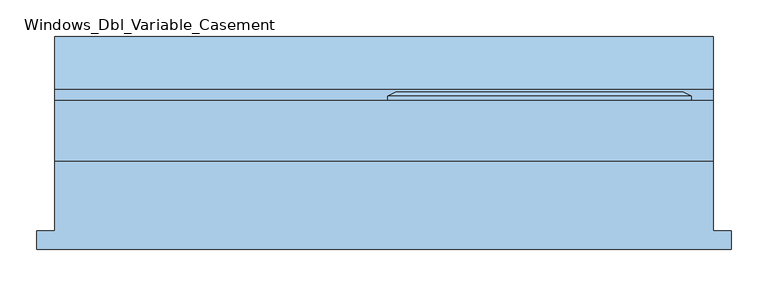
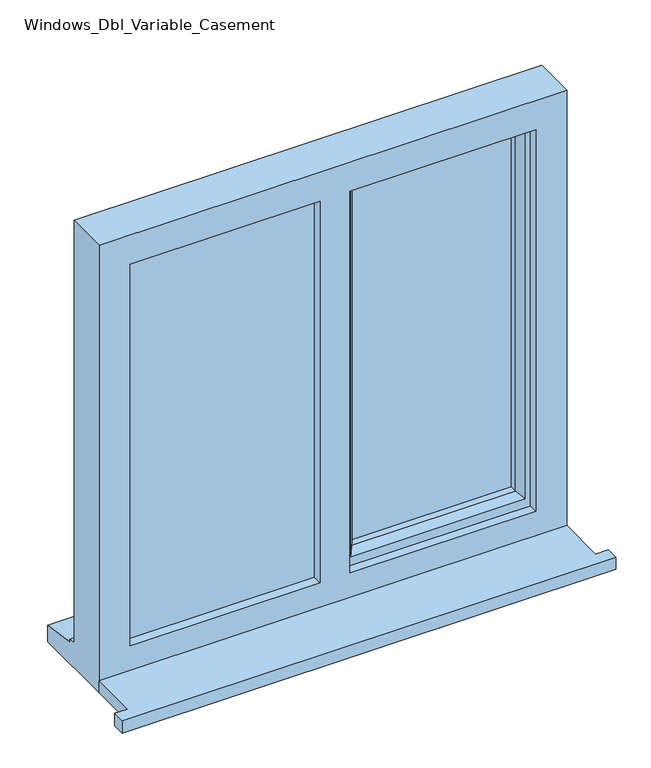
"""IFC4 building model written with IfcOpenShell, lengths in millimetres: window geometry, Windows_Dbl_Variable_Casement."""

from ifc_helpers import new_model, si_unit, frame, origin, place, context, project, spatial, polyline, outline, extrude, faceted_brep, source, transform, mapped, element, save


def windows_dbl_variable_casement_3235f540(model_context):
    return source(origin(), model_context, "Body", "SolidModel", [
        extrude(outline(polyline([(-760.0, -130.8434322), (-760.0, -105.8434322), (-735.0, -105.8434322), (-735.0, -10.2434322), (165.0, -10.2434322), (165.0, -105.8434322), (190.0, -105.8434322), (190.0, -130.8434322), (-760.0, -130.8434322)])), frame((0.0, 0.0, 1200.0), z_axis=(0.0, 0.0, 1.0), x_axis=(1.0, 0.0, 0.0)), (0.0, 0.0, 1.0), 25.0),
        faceted_brep([(-280.0, 72.7565678, 2080.0), (-280.0, 78.5300705, 2080.0), (-280.0, 78.5300705, 1253.0), (-280.0, 72.7565678, 1253.0), (-270.0, 7.7565678, 2070.0), (-270.0, 72.7565678, 2070.0), (-270.0, 72.7565678, 1263.0), (-270.0, 7.7565678, 1263.0), (-230.0, 22.2494677, 2030.0), (-240.1480377, 7.7565678, 2040.1480377), (-240.1480377, 7.7565678, 1292.8519623), (-230.0, 22.2494677, 1303.0), (-230.0, 36.7565678, 2030.0), (-230.0, 36.7565678, 1303.0), (-240.0, 60.7565678, 2040.0), (-240.0, 36.7565678, 2040.0), (-240.0, 36.7565678, 1293.0), (-240.0, 60.7565678, 1293.0), (-230.0, 78.5300705, 2030.0), (-230.0, 60.7565678, 2030.0), (-230.0, 60.7565678, 1303.0), (-230.0, 78.5300705, 1303.0), (-247.4457548, 84.3035732, 2047.4457548), (-247.4457548, 84.3035732, 1285.5542452), (-269.2153903, 84.3035732, 2069.2153903), (-269.2153903, 84.3035732, 1263.7846097), (135.0, 78.5300705, 1253.0), (135.0, 72.7565678, 1253.0), (125.0, 72.7565678, 1263.0), (125.0, 7.7565678, 1263.0), (95.1480377, 7.7565678, 1292.8519623), (85.0, 22.2494677, 1303.0), (85.0, 36.7565678, 1303.0), (95.0, 36.7565678, 1293.0), (95.0, 60.7565678, 1293.0), (85.0, 60.7565678, 1303.0), (85.0, 78.5300705, 1303.0), (102.4457548, 84.3035732, 1285.5542452), (124.2153903, 84.3035732, 1263.7846097), (135.0, 78.5300705, 2080.0), (135.0, 72.7565678, 2080.0), (125.0, 72.7565678, 2070.0), (125.0, 7.7565678, 2070.0), (95.1480377, 7.7565678, 2040.1480377), (85.0, 22.2494677, 2030.0), (85.0, 36.7565678, 2030.0), (95.0, 36.7565678, 2040.0), (95.0, 60.7565678, 2040.0), (85.0, 60.7565678, 2030.0), (85.0, 78.5300705, 2030.0), (102.4457548, 84.3035732, 2047.4457548), (124.2153903, 84.3035732, 2069.2153903)], [[[0, 1, 2, 3]], [[4, 5, 6, 7]], [[8, 9, 10, 11]], [[12, 8, 11, 13]], [[14, 15, 16, 17]], [[18, 19, 20, 21]], [[22, 18, 21, 23]], [[1, 24, 25, 2]], [[3, 2, 26, 27]], [[7, 6, 28, 29]], [[11, 10, 30, 31]], [[13, 11, 31, 32]], [[17, 16, 33, 34]], [[21, 20, 35, 36]], [[23, 21, 36, 37]], [[2, 25, 38, 26]], [[27, 26, 39, 40]], [[29, 28, 41, 42]], [[31, 30, 43, 44]], [[32, 31, 44, 45]], [[34, 33, 46, 47]], [[36, 35, 48, 49]], [[37, 36, 49, 50]], [[26, 38, 51, 39]], [[40, 39, 1, 0]], [[3, 27, 40, 0], [5, 41, 28, 6]], [[42, 41, 5, 4]], [[7, 29, 42, 4], [9, 43, 30, 10]], [[44, 43, 9, 8]], [[45, 44, 8, 12]], [[15, 46, 33, 16], [13, 32, 45, 12]], [[47, 46, 15, 14]], [[17, 34, 47, 14], [19, 48, 35, 20]], [[49, 48, 19, 18]], [[50, 49, 18, 22]], [[24, 51, 38, 25], [23, 37, 50, 22]], [[39, 51, 24, 1]]]),
        extrude(outline(polyline([(2050.0, -310.0), (2070.0, -310.0), (2070.0, -695.0), (1263.0, -695.0), (1263.0, -310.0), (1283.0, -310.0), (1283.0, -675.0), (2050.0, -675.0), (2050.0, -310.0)])), frame((0.0, 31.7565678, 0.0), z_axis=(0.0, 1.0, 0.0), x_axis=(0.0, 0.0, 1.0)), (0.0, 0.0, 1.0), 41.0),
        faceted_brep([(165.0, -10.2434322, 2110.0), (-735.0, -10.2434322, 2110.0), (-735.0, -10.2434322, 1200.0), (165.0, -10.2434322, 1200.0), (105.0, -10.2434322, 2050.0), (105.0, -10.2434322, 1275.0), (-252.0, -10.2434322, 1275.0), (-252.0, -10.2434322, 2050.0), (-310.0, -10.2434322, 2050.0), (-310.0, -10.2434322, 1275.0), (-675.0, -10.2434322, 1275.0), (-675.0, -10.2434322, 2050.0), (-735.0, 72.7565678, 2110.0), (-735.0, 72.7565678, 1251.0), (-735.0, 87.7565678, 1249.68767), (-735.0, 87.7565678, 1244.7449676), (-735.0, 160.2565678, 1233.8088847), (-735.0, 160.2565678, 1200.0), (165.0, 72.7565678, 2110.0), (165.0, 72.7565678, 1251.0), (-695.0, 72.7565678, 2070.0), (-695.0, 72.7565678, 1263.0), (-310.0, 72.7565678, 1263.0), (-310.0, 72.7565678, 2070.0), (-270.0, 72.7565678, 2070.0), (-270.0, 72.7565678, 1263.0), (125.0, 72.7565678, 1263.0), (125.0, 72.7565678, 2070.0), (-695.0, 7.7565678, 2070.0), (-695.0, 7.7565678, 1263.0), (-300.0, 7.7565678, 2070.0), (-300.0, 7.7565678, 1263.0), (-310.0, 7.7565678, 2050.0), (-675.0, 7.7565678, 2050.0), (-675.0, 7.7565678, 1275.0), (-310.0, 7.7565678, 1275.0), (-270.0, 7.7565678, 2070.0), (125.0, 7.7565678, 2070.0), (125.0, 7.7565678, 1263.0), (-270.0, 7.7565678, 1263.0), (105.0, 7.7565678, 2050.0), (-252.0, 7.7565678, 2050.0), (-252.0, 7.7565678, 1275.0), (105.0, 7.7565678, 1275.0), (-310.0, 31.7565678, 2070.0), (-300.0, 31.7565678, 2070.0), (165.0, 160.2565678, 1200.0), (165.0, 160.2565678, 1233.8088847), (165.0, 87.7565678, 1244.7449676), (165.0, 87.7565678, 1249.68767), (-300.0, 31.7565678, 1263.0), (-310.0, 31.7565678, 1263.0)], [[[0, 1, 2, 3], [4, 5, 6, 7], [8, 9, 10, 11]], [[2, 1, 12, 13, 14, 15, 16, 17]], [[13, 12, 18, 19], [20, 21, 22, 23], [24, 25, 26, 27]], [[21, 20, 28, 29]], [[28, 30, 31, 29], [32, 33, 34, 35]], [[36, 37, 38, 39], [40, 41, 42, 43]], [[33, 11, 10, 34]], [[1, 0, 18, 12]], [[28, 20, 23, 44, 45, 30]], [[27, 37, 36, 24]], [[11, 33, 32, 8]], [[40, 4, 7, 41]], [[19, 18, 0, 3, 46, 47, 48, 49]], [[27, 26, 38, 37]], [[4, 40, 43, 5]], [[45, 50, 31, 30]], [[50, 45, 44, 51]], [[51, 44, 23, 22]], [[25, 24, 36, 39]], [[41, 7, 6, 42]], [[8, 32, 35, 9]], [[46, 3, 2, 17]], [[47, 46, 17, 16]], [[48, 47, 16, 15]], [[49, 48, 15, 14]], [[19, 49, 14, 13]], [[22, 21, 29, 31, 50, 51]], [[26, 25, 39, 38]], [[6, 5, 43, 42]], [[35, 34, 10, 9]]]),
        extrude(outline(polyline([(-695.0, 31.7565678), (-300.0, 31.7565678), (-300.0, 7.7565678), (-695.0, 7.7565678), (-695.0, 31.7565678)])), frame((0.0, 0.0, 1263.0), z_axis=(0.0, 0.0, 1.0), x_axis=(1.0, 0.0, 0.0)), (0.0, 0.0, 1.0), 807.0),
        extrude(outline(polyline([(95.0, 36.7565678), (-240.0, 36.7565678), (-240.0, 60.7565678), (95.0, 60.7565678), (95.0, 36.7565678)])), frame((0.0, 0.0, 1293.0), z_axis=(0.0, 0.0, 1.0), x_axis=(1.0, 0.0, 0.0)), (0.0, 0.0, 1.0), 747.0),
    ])


if __name__ == "__main__":
    model = new_model("IFC4")
    model_context = context("Model", 3, world=origin())
    ifc_project = project(units=[si_unit("LENGTHUNIT", "METRE", prefix="MILLI")], contexts=[model_context])
    site = spatial("IfcSite", under=ifc_project)
    building = spatial("IfcBuilding", under=site)
    placement = place(None, origin())
    windows_dbl_variable_casement_shape = windows_dbl_variable_casement_3235f540(model_context)
    element("IfcWindow", 1, ObjectType="Windows_Dbl_Variable_Casement", at=placement, inside=building, context=model_context, shape_type="MappedRepresentation", body=[
        mapped(windows_dbl_variable_casement_shape, transform((0.0, 0.0, 0.0), x_axis=(1.0, 0.0, 0.0), y_axis=(0.0, 1.0, 0.0), z_axis=(0.0, 0.0, 1.0))),
    ])
    save(model, "model.ifc")

# Revit data of these elements
# Type "Windows_Dbl_Variable_Casement"
#   Type Mark = "58"
#   Operation = "DoublePanelVertical"
#   Construction Type Id = "GSP4R"
#   Manufacturer = "Revit"
#   Keynote = "L10"
#   Analytic Construction = "1/8 in Pilkington single glazing"
#   Wrap Layers (Int) from Ext = 0.1775 m
#   Wrap Layers (Ext) from Ext = 0.1025 m
#   Window Board Projection = 0.025 m
#   Window Board Extension = 0.025 m
#   Visual Light Transmittance = 0.9
#   Solar Heat Gain Coefficient = 0.78
#   Rough Width = 0.9 m
#   Rough Height = 0.91 m
#   Height = 0.91 m
#   Width = 0.9 m
#   Heat Transfer Coefficient (U) = 3.6886 W/(m²·K)
#   Glazing Thickness = 0.024 m
#   FrameOffset - External = 0.05 m
#   Frame Depth = 0.065 m
#   Default Head Height = 2.11 m
#   Cill Depth = 0.0875 m
#   Cavity Closer Width = 0.05 m
#   Cavity Closer Offset from Ext = 0.1025 m
#   Cavity Closer Depth = 0.085 m
#   Casement Width = 0.45 m
#   Vis - Cavity Closers = yes
#   Define Thermal Properties by = 1
#   Material Trim = Window Frame
#   Material Glass = Glass
#   Material Frame = Window Frame
#   Wall Closure = (empty or 0)
# Element 1 (IfcWindow, "Windows_Dbl_Variable_Casement")
#   Materials on its faces: "Window Frame", "Glass"
# Materials
#   "Window Frame": colour RGB 249 249 249, transparency 0, Keynote = "L10", Cost = 0
#   "Glass": class "Glass", colour RGB 0 128 192, transparency 0.9, Description = "Soda Lime Glass", Cost = 0
